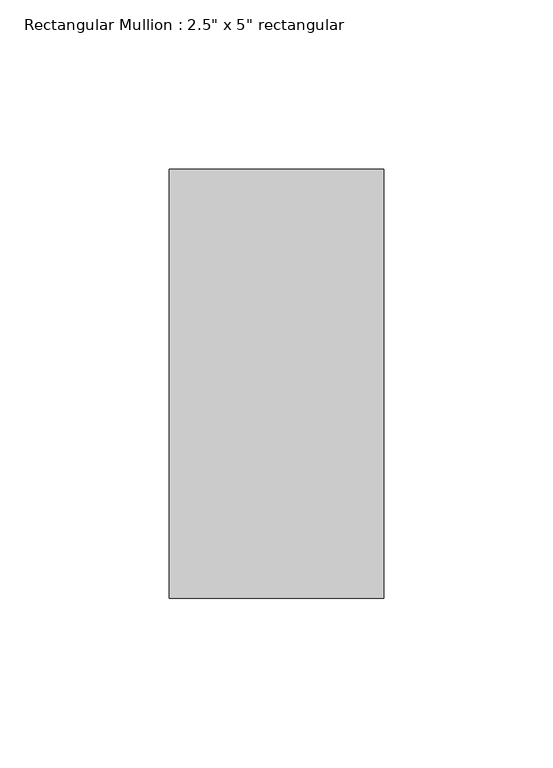
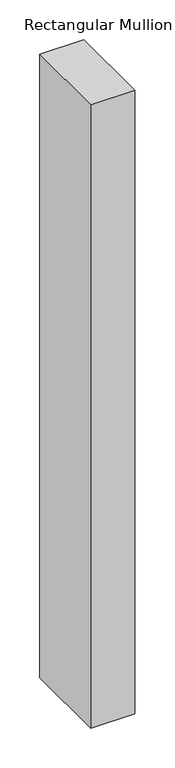
"""IFC4 building model written with IfcOpenShell, lengths in millimetres: member geometry."""

from ifc_helpers import new_model, si_unit, frame, origin, place, context, project, spatial, polyline, outline, extrude, source, transform, mapped, element, save


def member_194e59d8(model_context):
    return source(origin(), model_context, "Body", "SweptSolid", [
        extrude(outline(polyline([(0.0, 63.5), (0.0, -63.5), (-63.5, -63.5), (-63.5, 63.5), (0.0, 63.5)])), frame((0.0, 0.0, -952.5), z_axis=(0.0, 0.0, 1.0), x_axis=(1.0, 0.0, 0.0)), (0.0, 0.0, 1.0), 952.5),
    ])


if __name__ == "__main__":
    model = new_model("IFC4")
    model_context = context("Model", 3, world=origin())
    ifc_project = project(units=[si_unit("LENGTHUNIT", "METRE", prefix="MILLI")], contexts=[model_context])
    site = spatial("IfcSite", under=ifc_project)
    building = spatial("IfcBuilding", under=site)
    placement = place(None, origin())
    member_shape = member_194e59d8(model_context)
    element("IfcMember", 1, ObjectType="Rectangular Mullion : 2.5\" x 5\" rectangular", at=placement, inside=building, context=model_context, shape_type="MappedRepresentation", body=[
        mapped(member_shape, transform((0.0, 0.0, 0.0), x_axis=(1.0, 0.0, 0.0), y_axis=(0.0, 1.0, 0.0), z_axis=(0.0, 0.0, 1.0))),
    ])
    save(model, "model.ifc")

# Revit data of these elements
# Type "Rectangular Mullion : 2.5\" x 5\" rectangular"
#   built-in parameter 1007304 = 0.416667 (stored number, unit not read)
#   built-in parameter 1007301 = 0.104167 (stored number, unit not read)
#   built-in parameter 1007300 = 0.104167 (stored number, unit not read)
# Element 1 (IfcMember, "Rectangular Mullion : 2.5\" x 5\" rectangular")
#   Materials on its faces: "Aluminum"
# Materials
#   "Aluminum": class "Metal", colour RGB 247 247 247, transparency 0, Description = "Aluminum 6061", Cost = 0
